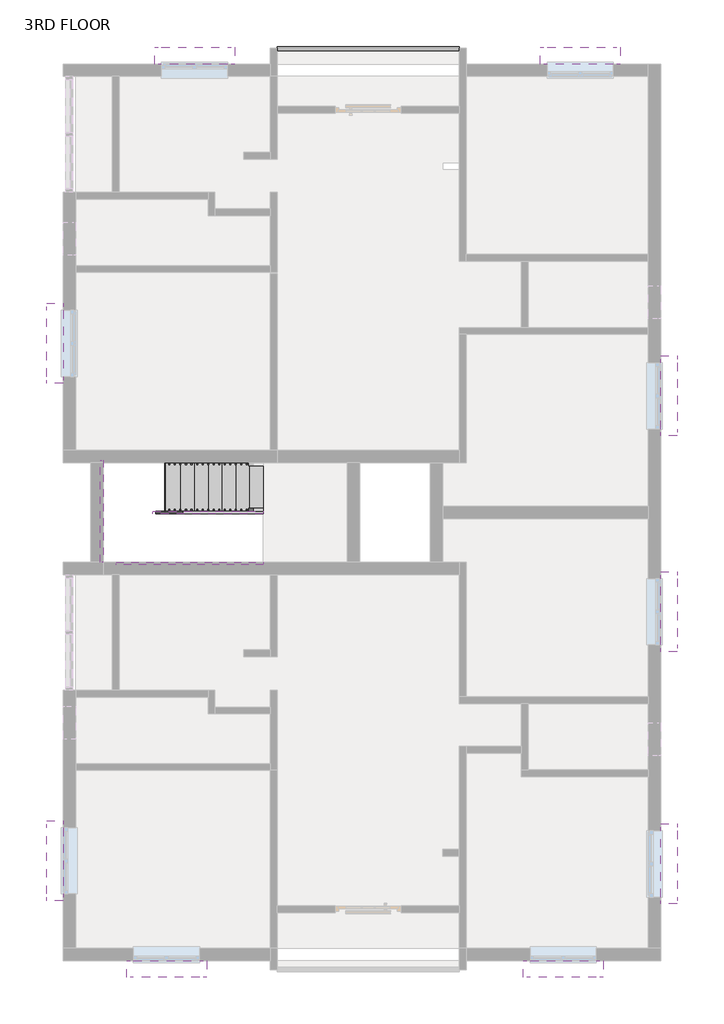
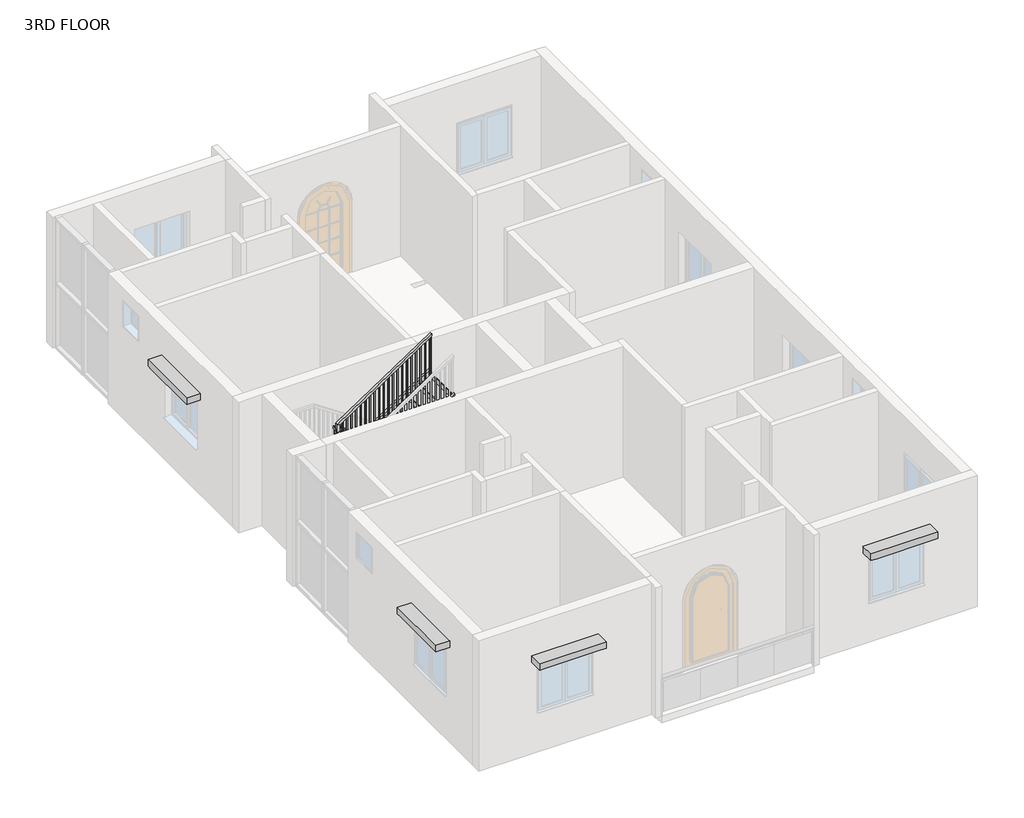
# One storey, part 4 of 4: 9 proxies, 5 members, 2 railings, 1 stair flight.
"""IFC4 building model written with IfcOpenShell, lengths in millimetres."""

from ifc_helpers import new_model, si_unit, point, frame, origin, place, context, project, spatial, polyline, ellipse_curve, trimmed, outline, extrude, faceted_brep, transform, mapped, element, save
from ifc_brep_helpers import plane_surface, extruded_surface, advanced_brep
from components import generic_models_11_generic_models_11_d301a5e8, generic_models_21_generic_models_21_87948dc1, generic_models_1_generic_models_1_fbb7ad13, generic_models_36_generic_models_36_9c63594f, stair_flight_d3eadeea

model = new_model("IFC4")

# Units and contexts
model_context = context("Model", 3, world=origin())
ifc_project = project(units=[si_unit("LENGTHUNIT", "METRE", prefix="MILLI")], contexts=[model_context])

# Site, building, storey
site = spatial("IfcSite", under=ifc_project)
building = spatial("IfcBuilding", under=site)
storey = spatial("IfcBuildingStorey", under=building, Name="3RD FLOOR", Elevation=12192.0)

# Proxies
placement = place(None, origin())
generic_models_11_generic_models_11_shape = generic_models_11_generic_models_11_d301a5e8(model_context)
element("IfcBuildingElementProxy", 1, Name="Generic Models 13 : Generic Models 11", ObjectType="Generic Models 13 : Generic Models 11", at=placement, inside=storey, context=model_context, shape_type="MappedRepresentation", body=[
    mapped(generic_models_11_generic_models_11_shape, transform((0.0, 0.0, -3048.0), x_axis=(1.0, 0.0, 0.0), y_axis=(0.0, 1.0, 0.0), z_axis=(0.0, 0.0, 1.0))),
])
element("IfcBuildingElementProxy", 2, Name="Generic Models 14 : Generic Models 11", ObjectType="Generic Models 14 : Generic Models 11", at=placement, inside=storey, context=model_context, shape_type="MappedRepresentation", body=[
    mapped(generic_models_11_generic_models_11_shape, transform((-7101.0359618, 0.0, -3048.0), x_axis=(1.0, 0.0, 0.0), y_axis=(0.0, 1.0, 0.0), z_axis=(0.0, 0.0, 1.0))),
])
generic_models_21_generic_models_21_shape = generic_models_21_generic_models_21_87948dc1(model_context)
element("IfcBuildingElementProxy", 3, Name="Generic Models 24 : Generic Models 21", ObjectType="Generic Models 24 : Generic Models 21", at=placement, inside=storey, context=model_context, shape_type="MappedRepresentation", body=[
    mapped(generic_models_21_generic_models_21_shape, transform((0.0, 0.0, -3048.0), x_axis=(1.0, 0.0, 0.0), y_axis=(0.0, 1.0, 0.0), z_axis=(0.0, 0.0, 1.0))),
])
element("IfcBuildingElementProxy", 4, Name="Generic Models 25 : Generic Models 21", ObjectType="Generic Models 25 : Generic Models 21", at=placement, inside=storey, context=model_context, shape_type="MappedRepresentation", body=[
    mapped(generic_models_21_generic_models_21_shape, transform((0.0, 4641.85, -3133.6), x_axis=(1.0, 0.0, 0.0), y_axis=(0.0, 1.0, 0.0), z_axis=(0.0, 0.0, 1.0))),
])
element("IfcBuildingElementProxy", 5, Name="Generic Models 26 : Generic Models 21", ObjectType="Generic Models 26 : Generic Models 21", at=placement, inside=storey, context=model_context, shape_type="MappedRepresentation", body=[
    mapped(generic_models_21_generic_models_21_shape, transform((0.0, 8616.95, -3133.6), x_axis=(1.0, 0.0, 0.0), y_axis=(0.0, 1.0, 0.0), z_axis=(0.0, 0.0, 1.0))),
])
generic_models_1_generic_models_1_shape = generic_models_1_generic_models_1_fbb7ad13(model_context)
element("IfcBuildingElementProxy", 6, Name="Generic Models 3 : Generic Models 1", ObjectType="Generic Models 3 : Generic Models 1", at=placement, inside=storey, context=model_context, shape_type="MappedRepresentation", body=[
    mapped(generic_models_1_generic_models_1_shape, transform((0.0, 0.0, -3048.0), x_axis=(1.0, 0.0, 0.0), y_axis=(0.0, 1.0, 0.0), z_axis=(0.0, 0.0, 1.0))),
])
generic_models_36_generic_models_36_shape = generic_models_36_generic_models_36_9c63594f(model_context)
element("IfcBuildingElementProxy", 7, Name="Generic Models 38 : Generic Models 36", ObjectType="Generic Models 38 : Generic Models 36", at=placement, inside=storey, context=model_context, shape_type="MappedRepresentation", body=[
    mapped(generic_models_36_generic_models_36_shape, transform((0.0, 0.0, -3048.0), x_axis=(1.0, 0.0, 0.0), y_axis=(0.0, 1.0, 0.0), z_axis=(0.0, 0.0, 1.0))),
])
element("IfcBuildingElementProxy", 8, Name="Generic Models 39 : Generic Models 36", ObjectType="Generic Models 39 : Generic Models 36", at=placement, inside=storey, context=model_context, shape_type="MappedRepresentation", body=[
    mapped(generic_models_36_generic_models_36_shape, transform((0.0, -9525.0, -3048.0), x_axis=(1.0, 0.0, 0.0), y_axis=(0.0, 1.0, 0.0), z_axis=(0.0, 0.0, 1.0))),
])
element("IfcBuildingElementProxy", 9, Name="Generic Models 4 : Generic Models 1", ObjectType="Generic Models 4 : Generic Models 1", at=placement, inside=storey, context=model_context, shape_type="MappedRepresentation", body=[
    mapped(generic_models_1_generic_models_1_shape, transform((7304.0875, 0.0, -3048.0), x_axis=(1.0, 0.0, 0.0), y_axis=(0.0, 1.0, 0.0), z_axis=(0.0, 0.0, 1.0))),
])

# Members
element("IfcMember", 10, ObjectType="Stringer - 2\" Width", at=placement, inside=storey, context=model_context, shape_type="SweptSolid", body=[
    extrude(outline(polyline([(12192.0, -2748.0012202), (12410.0398409, -2748.0012202), (13730.8398409, -4729.2012202), (13364.5158313, -4729.2012202), (12192.0, -2970.4274732), (12192.0, -2748.0012202)])), frame((0.0, 4990.8309003, 0.0), z_axis=(0.0, 1.0, 0.0), x_axis=(0.0, 0.0, 1.0)), (0.0, 0.0, 1.0), 50.8),
])
element("IfcMember", 11, ObjectType="Stringer - 2\" Width", at=placement, inside=storey, context=model_context, shape_type="SweptSolid", body=[
    extrude(outline(polyline([(13934.0398409, -4780.0012202), (13567.7158313, -4780.0012202), (14922.382498, -2748.0012202), (15288.7065076, -2748.0012202), (13934.0398409, -4780.0012202)])), frame((0.0, 4990.8309003, 0.0), z_axis=(0.0, 1.0, 0.0), x_axis=(0.0, 0.0, 1.0)), (0.0, 0.0, 1.0), 50.8),
])
element("IfcMember", 12, ObjectType="Stringer - 2\" Width", at=placement, inside=storey, context=model_context, shape_type="SweptSolid", body=[
    extrude(outline(polyline([(12192.0, -2748.0012202), (12410.0398409, -2748.0012202), (13792.2, -4821.2414588), (13792.2, -5370.7274732), (12192.0, -2970.4274732), (12192.0, -2748.0012202)])), frame((0.0, 5930.6309003, 0.0), z_axis=(0.0, 1.0, 0.0), x_axis=(0.0, 0.0, 1.0)), (0.0, 0.0, 1.0), 50.8),
])
element("IfcMember", 13, ObjectType="Stringer - 2\" Width", at=placement, inside=storey, context=model_context, shape_type="SweptSolid", body=[
    extrude(outline(polyline([(-5745.2012202, 5981.4309003), (-5694.4012202, 5981.4309003), (-5694.4012202, 4101.8309003), (-5745.2012202, 4101.8309003), (-5745.2012202, 5981.4309003)])), frame((0.0, 0.0, 13487.4), z_axis=(0.0, 0.0, 1.0), x_axis=(1.0, 0.0, 0.0)), (0.0, 0.0, 1.0), 304.8),
])
element("IfcMember", 14, ObjectType="Stringer - 2\" Width", at=placement, inside=storey, context=model_context, shape_type="SweptSolid", body=[
    extrude(outline(polyline([(13487.4, -4900.4749672), (14922.382498, -2748.0012202), (15288.7065076, -2748.0012202), (13487.4, -5449.9609815), (13487.4, -4900.4749672)])), frame((0.0, 4051.0309003, 0.0), z_axis=(0.0, 1.0, 0.0), x_axis=(0.0, 0.0, 1.0)), (0.0, 0.0, 1.0), 50.8),
])

# Railings
element("IfcRailing", 15, ObjectType="Glass Panel - Bottom Fill 2", at=placement, inside=storey, context=model_context, shape_type="SolidModel", body=[
    advanced_brep(
    [(-2494.0012202, 13593.7910566, 13106.4), (-2494.0012202, 13517.5910566, 13106.4), (858.7987798, 13593.7910566, 13106.4), (858.7987798, 13517.5910566, 13106.4)],
    [
        (0, 1, ellipse_curve(frame((-2494.0012202, 13555.6910566, 13106.4), z_axis=(-1.0, 0.0, 0.0), x_axis=(0.0, -1.0, 0.0)), 38.1, 28.575)),
        (1, 0, ellipse_curve(frame((-2494.0012202, 13555.6910566, 13106.4), z_axis=(-1.0, 0.0, 0.0), x_axis=(0.0, -1.0, 0.0)), 38.1, 28.575)),
        (2, 3, ellipse_curve(frame((858.7987798, 13555.6910566, 13106.4), z_axis=(1.0, 0.0, 0.0), x_axis=(0.0, -1.0, 0.0)), 38.1, 28.575)),
        (3, 2, ellipse_curve(frame((858.7987798, 13555.6910566, 13106.4), z_axis=(1.0, 0.0, 0.0), x_axis=(0.0, -1.0, 0.0)), 38.1, 28.575)),
        (0, 2),
        (3, 1),
    ],
    [
        plane_surface(frame((-2494.0012202, 13555.6910566, 13106.4), z_axis=(-1.0, 0.0, 0.0), x_axis=(0.0, 1.0, 0.0))),
        plane_surface(frame((858.7987798, 13555.6910566, 13106.4), z_axis=(1.0, 0.0, 0.0), x_axis=(0.0, 1.0, 0.0))),
        extruded_surface(trimmed(ellipse_curve(frame((858.7987798, 13555.6910566, 13106.4), z_axis=(-1.0, 0.0, 0.0), x_axis=(0.0, -1.0, 0.0)), 38.1, 28.575), [point((858.7987798, 13593.7910566, 13106.4))], [point((858.7987798, 13517.5910566, 13106.4))], True, "CARTESIAN"), (-3352.7999999999997, 0.0, 0.0), 3352.7999999999997),
        extruded_surface(trimmed(ellipse_curve(frame((858.7987798, 13555.6910566, 13106.4), z_axis=(-1.0, 0.0, 0.0), x_axis=(0.0, -1.0, 0.0)), 38.1, 28.575), [point((858.7987798, 13517.5910566, 13106.4))], [point((858.7987798, 13593.7910566, 13106.4))], True, "CARTESIAN"), (-3352.7999999999997, 0.0, 0.0), 3352.7999999999997),
    ],
    [
        (0, [[1, 2]]),
        (1, [[3, 4]]),
        (2, [[-1, 5, -4, 6]]),
        (3, [[-2, -6, -3, -5]]),
    ],
),
    extrude(outline(polyline([(-4.8012202, 13562.2262136), (807.9987798, 13562.2262136), (807.9987798, 13555.8762136), (-4.8012202, 13555.8762136), (-4.8012202, 13562.2262136)])), frame((0.0, 0.0, 12293.6), z_axis=(0.0, 0.0, 1.0), x_axis=(1.0, 0.0, 0.0)), (0.0, 0.0, 1.0), 711.2),
    extrude(outline(polyline([(-817.6012202, 13562.2262136), (-4.8012202, 13562.2262136), (-4.8012202, 13555.8762136), (-817.6012202, 13555.8762136), (-817.6012202, 13562.2262136)])), frame((0.0, 0.0, 12293.6), z_axis=(0.0, 0.0, 1.0), x_axis=(1.0, 0.0, 0.0)), (0.0, 0.0, 1.0), 711.2),
    extrude(outline(polyline([(-1630.4012202, 13562.2262136), (-817.6012202, 13562.2262136), (-817.6012202, 13555.8762136), (-1630.4012202, 13555.8762136), (-1630.4012202, 13562.2262136)])), frame((0.0, 0.0, 12293.6), z_axis=(0.0, 0.0, 1.0), x_axis=(1.0, 0.0, 0.0)), (0.0, 0.0, 1.0), 711.2),
    extrude(outline(polyline([(-2443.2012202, 13562.2262136), (-1630.4012202, 13562.2262136), (-1630.4012202, 13555.8762136), (-2443.2012202, 13555.8762136), (-2443.2012202, 13562.2262136)])), frame((0.0, 0.0, 12293.6), z_axis=(0.0, 0.0, 1.0), x_axis=(1.0, 0.0, 0.0)), (0.0, 0.0, 1.0), 711.2),
    extrude(outline(polyline([(846.0987798, 13546.1660566), (846.0987798, 13565.2160566), (865.1487798, 13565.2160566), (865.1487798, 13546.1660566), (846.0987798, 13546.1660566)])), frame((0.0, 0.0, 12192.0), z_axis=(0.0, 0.0, 1.0), x_axis=(1.0, 0.0, 0.0)), (0.0, 0.0, 1.0), 885.825),
    extrude(outline(polyline([(-2500.3512202, 13546.1660566), (-2500.3512202, 13565.2160566), (-2481.3012202, 13565.2160566), (-2481.3012202, 13546.1660566), (-2500.3512202, 13546.1660566)])), frame((0.0, 0.0, 12192.0), z_axis=(0.0, 0.0, 1.0), x_axis=(1.0, 0.0, 0.0)), (0.0, 0.0, 1.0), 885.825),
])
element("IfcRailing", 16, ObjectType="Handrail - Rectangular", at=placement, inside=storey, context=model_context, shape_type="SolidModel", body=[
    faceted_brep([(-2748.0012202, 5041.6309003, 13275.7333333), (-2748.0012202, 5041.6309003, 13214.6793317), (-2748.0012202, 5092.4309003, 13214.6793317), (-2748.0012202, 5092.4309003, 13275.7333333), (-4703.8012202, 5041.6309003, 14579.6), (-4754.6012202, 5041.6309003, 14552.4126651), (-4754.6012202, 5092.4309003, 14552.4126651), (-4703.8012202, 5092.4309003, 14579.6), (-4703.8012202, 5041.6309003, 14630.4), (-4754.6012202, 5041.6309003, 14579.6), (-4754.6012202, 5092.4309003, 14579.6), (-4703.8012202, 5092.4309003, 14630.4), (-4780.0012202, 5041.6309003, 14630.4), (-4780.0012202, 5041.6309003, 14579.6), (-4830.8012202, 5092.4309003, 14579.6), (-4830.8012202, 5092.4309003, 14630.4), (-4780.0012202, 4990.8309003, 14630.4), (-4830.8012202, 4990.8309003, 14630.4), (-4830.8012202, 4940.0309003, 14579.6), (-4780.0012202, 4940.0309003, 14579.6)], [[[0, 1, 2, 3]], [[1, 0, 4, 5]], [[2, 1, 5, 6]], [[3, 2, 6, 7]], [[0, 3, 7, 4]], [[5, 4, 8, 9]], [[6, 5, 9, 10]], [[7, 6, 10, 11]], [[4, 7, 11, 8]], [[9, 8, 12, 13]], [[10, 9, 13, 14]], [[11, 10, 14, 15]], [[8, 11, 15, 12]], [[16, 17, 18, 19]], [[13, 12, 16, 19]], [[14, 13, 19, 18]], [[15, 14, 18, 17]], [[12, 15, 17, 16]]]),
    faceted_brep([(-4780.0012202, 4990.8309003, 14630.4), (-4780.0012202, 4940.0309003, 14579.6), (-4830.8012202, 4940.0309003, 14579.6), (-4830.8012202, 4990.8309003, 14630.4), (-4780.0012202, 4990.8309003, 14738.6793317), (-4830.8012202, 4990.8309003, 14765.8666667), (-4830.8012202, 4940.0309003, 14765.8666667), (-4780.0012202, 4940.0309003, 14738.6793317)], [[[0, 1, 2, 3]], [[4, 5, 6, 7]], [[1, 0, 4, 7]], [[2, 1, 7, 6]], [[3, 2, 6, 5]], [[0, 3, 5, 4]]]),
    faceted_brep([(-4830.8012202, 4990.8309003, 14765.8666667), (-4780.0012202, 4990.8309003, 14738.6793317), (-4780.0012202, 4940.0309003, 14738.6793317), (-4830.8012202, 4940.0309003, 14765.8666667), (-2748.0012202, 4990.8309003, 16154.4), (-2748.0012202, 4940.0309003, 16154.4), (-2748.0012202, 4940.0309003, 16093.3459984), (-2748.0012202, 4990.8309003, 16093.3459984)], [[[0, 1, 2, 3]], [[4, 5, 6, 7]], [[1, 0, 4, 7]], [[2, 1, 7, 6]], [[3, 2, 6, 5]], [[0, 3, 5, 4]]]),
    extrude(outline(polyline([(16070.0626651, -2782.9262202), (15070.6666667, -2782.9262202), (15070.6666667, -2763.8762202), (16082.7626651, -2763.8762202), (16070.0626651, -2782.9262202)])), frame((0.0, 4955.9059003, 0.0), z_axis=(0.0, 1.0, 0.0), x_axis=(0.0, 0.0, 1.0)), (0.0, 0.0, 1.0), 19.05),
    extrude(outline(polyline([(16002.3293317, -2884.5262202), (15070.6666667, -2884.5262202), (15070.6666667, -2865.4762202), (16015.0293317, -2865.4762202), (16002.3293317, -2884.5262202)])), frame((0.0, 4955.9059003, 0.0), z_axis=(0.0, 1.0, 0.0), x_axis=(0.0, 0.0, 1.0)), (0.0, 0.0, 1.0), 19.05),
    extrude(outline(polyline([(15934.5959984, -2986.1262202), (15070.6666667, -2986.1262202), (15070.6666667, -2967.0762202), (15947.2959984, -2967.0762202), (15934.5959984, -2986.1262202)])), frame((0.0, 4955.9059003, 0.0), z_axis=(0.0, 1.0, 0.0), x_axis=(0.0, 0.0, 1.0)), (0.0, 0.0, 1.0), 19.05),
    extrude(outline(polyline([(15866.8626651, -3087.7262202), (14901.3333333, -3087.7262202), (14901.3333333, -3068.6762202), (15879.5626651, -3068.6762202), (15866.8626651, -3087.7262202)])), frame((0.0, 4955.9059003, 0.0), z_axis=(0.0, 1.0, 0.0), x_axis=(0.0, 0.0, 1.0)), (0.0, 0.0, 1.0), 19.05),
    extrude(outline(polyline([(15799.1293317, -3189.3262202), (14901.3333333, -3189.3262202), (14901.3333333, -3170.2762202), (15811.8293317, -3170.2762202), (15799.1293317, -3189.3262202)])), frame((0.0, 4955.9059003, 0.0), z_axis=(0.0, 1.0, 0.0), x_axis=(0.0, 0.0, 1.0)), (0.0, 0.0, 1.0), 19.05),
    extrude(outline(polyline([(15731.3959984, -3290.9262202), (14732.0, -3290.9262202), (14732.0, -3271.8762202), (15744.0959984, -3271.8762202), (15731.3959984, -3290.9262202)])), frame((0.0, 4955.9059003, 0.0), z_axis=(0.0, 1.0, 0.0), x_axis=(0.0, 0.0, 1.0)), (0.0, 0.0, 1.0), 19.05),
    extrude(outline(polyline([(15663.6626651, -3392.5262202), (14732.0, -3392.5262202), (14732.0, -3373.4762202), (15676.3626651, -3373.4762202), (15663.6626651, -3392.5262202)])), frame((0.0, 4955.9059003, 0.0), z_axis=(0.0, 1.0, 0.0), x_axis=(0.0, 0.0, 1.0)), (0.0, 0.0, 1.0), 19.05),
    extrude(outline(polyline([(15595.9293317, -3494.1262202), (14732.0, -3494.1262202), (14732.0, -3475.0762202), (15608.6293317, -3475.0762202), (15595.9293317, -3494.1262202)])), frame((0.0, 4955.9059003, 0.0), z_axis=(0.0, 1.0, 0.0), x_axis=(0.0, 0.0, 1.0)), (0.0, 0.0, 1.0), 19.05),
    extrude(outline(polyline([(15528.1959984, -3595.7262202), (14562.6666667, -3595.7262202), (14562.6666667, -3576.6762202), (15540.8959984, -3576.6762202), (15528.1959984, -3595.7262202)])), frame((0.0, 4955.9059003, 0.0), z_axis=(0.0, 1.0, 0.0), x_axis=(0.0, 0.0, 1.0)), (0.0, 0.0, 1.0), 19.05),
    extrude(outline(polyline([(15460.4626651, -3697.3262202), (14562.6666667, -3697.3262202), (14562.6666667, -3678.2762202), (15473.1626651, -3678.2762202), (15460.4626651, -3697.3262202)])), frame((0.0, 4955.9059003, 0.0), z_axis=(0.0, 1.0, 0.0), x_axis=(0.0, 0.0, 1.0)), (0.0, 0.0, 1.0), 19.05),
    extrude(outline(polyline([(15392.7293317, -3798.9262202), (14393.3333333, -3798.9262202), (14393.3333333, -3779.8762202), (15405.4293317, -3779.8762202), (15392.7293317, -3798.9262202)])), frame((0.0, 4955.9059003, 0.0), z_axis=(0.0, 1.0, 0.0), x_axis=(0.0, 0.0, 1.0)), (0.0, 0.0, 1.0), 19.05),
    extrude(outline(polyline([(15324.9959984, -3900.5262202), (14393.3333333, -3900.5262202), (14393.3333333, -3881.4762202), (15337.6959984, -3881.4762202), (15324.9959984, -3900.5262202)])), frame((0.0, 4955.9059003, 0.0), z_axis=(0.0, 1.0, 0.0), x_axis=(0.0, 0.0, 1.0)), (0.0, 0.0, 1.0), 19.05),
    extrude(outline(polyline([(15257.2626651, -4002.1262202), (14393.3333333, -4002.1262202), (14393.3333333, -3983.0762202), (15269.9626651, -3983.0762202), (15257.2626651, -4002.1262202)])), frame((0.0, 4955.9059003, 0.0), z_axis=(0.0, 1.0, 0.0), x_axis=(0.0, 0.0, 1.0)), (0.0, 0.0, 1.0), 19.05),
    extrude(outline(polyline([(15189.5293317, -4103.7262202), (14224.0, -4103.7262202), (14224.0, -4084.6762202), (15202.2293317, -4084.6762202), (15189.5293317, -4103.7262202)])), frame((0.0, 4955.9059003, 0.0), z_axis=(0.0, 1.0, 0.0), x_axis=(0.0, 0.0, 1.0)), (0.0, 0.0, 1.0), 19.05),
    extrude(outline(polyline([(15121.7959984, -4205.3262202), (14224.0, -4205.3262202), (14224.0, -4186.2762202), (15134.4959984, -4186.2762202), (15121.7959984, -4205.3262202)])), frame((0.0, 4955.9059003, 0.0), z_axis=(0.0, 1.0, 0.0), x_axis=(0.0, 0.0, 1.0)), (0.0, 0.0, 1.0), 19.05),
    extrude(outline(polyline([(15054.0626651, -4306.9262202), (14054.6666667, -4306.9262202), (14054.6666667, -4287.8762202), (15066.7626651, -4287.8762202), (15054.0626651, -4306.9262202)])), frame((0.0, 4955.9059003, 0.0), z_axis=(0.0, 1.0, 0.0), x_axis=(0.0, 0.0, 1.0)), (0.0, 0.0, 1.0), 19.05),
    extrude(outline(polyline([(14986.3293317, -4408.5262202), (14054.6666667, -4408.5262202), (14054.6666667, -4389.4762202), (14999.0293317, -4389.4762202), (14986.3293317, -4408.5262202)])), frame((0.0, 4955.9059003, 0.0), z_axis=(0.0, 1.0, 0.0), x_axis=(0.0, 0.0, 1.0)), (0.0, 0.0, 1.0), 19.05),
    extrude(outline(polyline([(14918.5959984, -4510.1262202), (14054.6666667, -4510.1262202), (14054.6666667, -4491.0762202), (14931.2959984, -4491.0762202), (14918.5959984, -4510.1262202)])), frame((0.0, 4955.9059003, 0.0), z_axis=(0.0, 1.0, 0.0), x_axis=(0.0, 0.0, 1.0)), (0.0, 0.0, 1.0), 19.05),
    extrude(outline(polyline([(14850.8626651, -4611.7262202), (13885.3333333, -4611.7262202), (13885.3333333, -4592.6762202), (14863.5626651, -4592.6762202), (14850.8626651, -4611.7262202)])), frame((0.0, 4955.9059003, 0.0), z_axis=(0.0, 1.0, 0.0), x_axis=(0.0, 0.0, 1.0)), (0.0, 0.0, 1.0), 19.05),
    extrude(outline(polyline([(14783.1293317, -4713.3262202), (13885.3333333, -4713.3262202), (13885.3333333, -4694.2762202), (14795.8293317, -4694.2762202), (14783.1293317, -4713.3262202)])), frame((0.0, 4955.9059003, 0.0), z_axis=(0.0, 1.0, 0.0), x_axis=(0.0, 0.0, 1.0)), (0.0, 0.0, 1.0), 19.05),
    extrude(outline(polyline([(-4770.4762202, 5057.5059003), (-4789.5262202, 5057.5059003), (-4789.5262202, 5076.5559003), (-4770.4762202, 5076.5559003), (-4770.4762202, 5057.5059003)])), frame((0.0, 0.0, 13716.0), z_axis=(0.0, 0.0, 1.0), x_axis=(1.0, 0.0, 0.0)), (0.0, 0.0, 1.0), 863.6),
    extrude(outline(polyline([(14507.9626651, -4687.9262202), (13546.6666667, -4687.9262202), (13546.6666667, -4668.8762202), (14495.2626651, -4668.8762202), (14507.9626651, -4687.9262202)])), frame((0.0, 5057.5059003, 0.0), z_axis=(0.0, 1.0, 0.0), x_axis=(0.0, 0.0, 1.0)), (0.0, 0.0, 1.0), 19.05),
    extrude(outline(polyline([(14440.2293317, -4586.3262202), (13546.6666667, -4586.3262202), (13546.6666667, -4567.2762202), (14427.5293317, -4567.2762202), (14440.2293317, -4586.3262202)])), frame((0.0, 5057.5059003, 0.0), z_axis=(0.0, 1.0, 0.0), x_axis=(0.0, 0.0, 1.0)), (0.0, 0.0, 1.0), 19.05),
    extrude(outline(polyline([(14372.4959984, -4484.7262202), (13377.3333333, -4484.7262202), (13377.3333333, -4465.6762202), (14359.7959984, -4465.6762202), (14372.4959984, -4484.7262202)])), frame((0.0, 5057.5059003, 0.0), z_axis=(0.0, 1.0, 0.0), x_axis=(0.0, 0.0, 1.0)), (0.0, 0.0, 1.0), 19.05),
    extrude(outline(polyline([(14304.7626651, -4383.1262202), (13377.3333333, -4383.1262202), (13377.3333333, -4364.0762202), (14292.0626651, -4364.0762202), (14304.7626651, -4383.1262202)])), frame((0.0, 5057.5059003, 0.0), z_axis=(0.0, 1.0, 0.0), x_axis=(0.0, 0.0, 1.0)), (0.0, 0.0, 1.0), 19.05),
    extrude(outline(polyline([(14237.0293317, -4281.5262202), (13377.3333333, -4281.5262202), (13377.3333333, -4262.4762202), (14224.3293317, -4262.4762202), (14237.0293317, -4281.5262202)])), frame((0.0, 5057.5059003, 0.0), z_axis=(0.0, 1.0, 0.0), x_axis=(0.0, 0.0, 1.0)), (0.0, 0.0, 1.0), 19.05),
    extrude(outline(polyline([(14169.2959984, -4179.9262202), (13208.0, -4179.9262202), (13208.0, -4160.8762202), (14156.5959984, -4160.8762202), (14169.2959984, -4179.9262202)])), frame((0.0, 5057.5059003, 0.0), z_axis=(0.0, 1.0, 0.0), x_axis=(0.0, 0.0, 1.0)), (0.0, 0.0, 1.0), 19.05),
    extrude(outline(polyline([(14101.5626651, -4078.3262202), (13208.0, -4078.3262202), (13208.0, -4059.2762202), (14088.8626651, -4059.2762202), (14101.5626651, -4078.3262202)])), frame((0.0, 5057.5059003, 0.0), z_axis=(0.0, 1.0, 0.0), x_axis=(0.0, 0.0, 1.0)), (0.0, 0.0, 1.0), 19.05),
    extrude(outline(polyline([(14033.8293317, -3976.7262202), (13038.6666667, -3976.7262202), (13038.6666667, -3957.6762202), (14021.1293317, -3957.6762202), (14033.8293317, -3976.7262202)])), frame((0.0, 5057.5059003, 0.0), z_axis=(0.0, 1.0, 0.0), x_axis=(0.0, 0.0, 1.0)), (0.0, 0.0, 1.0), 19.05),
    extrude(outline(polyline([(13966.0959984, -3875.1262202), (13038.6666667, -3875.1262202), (13038.6666667, -3856.0762202), (13953.3959984, -3856.0762202), (13966.0959984, -3875.1262202)])), frame((0.0, 5057.5059003, 0.0), z_axis=(0.0, 1.0, 0.0), x_axis=(0.0, 0.0, 1.0)), (0.0, 0.0, 1.0), 19.05),
    extrude(outline(polyline([(13898.3626651, -3773.5262202), (13038.6666667, -3773.5262202), (13038.6666667, -3754.4762202), (13885.6626651, -3754.4762202), (13898.3626651, -3773.5262202)])), frame((0.0, 5057.5059003, 0.0), z_axis=(0.0, 1.0, 0.0), x_axis=(0.0, 0.0, 1.0)), (0.0, 0.0, 1.0), 19.05),
    extrude(outline(polyline([(13830.6293317, -3671.9262202), (12869.3333333, -3671.9262202), (12869.3333333, -3652.8762202), (13817.9293317, -3652.8762202), (13830.6293317, -3671.9262202)])), frame((0.0, 5057.5059003, 0.0), z_axis=(0.0, 1.0, 0.0), x_axis=(0.0, 0.0, 1.0)), (0.0, 0.0, 1.0), 19.05),
    extrude(outline(polyline([(13762.8959984, -3570.3262202), (12869.3333333, -3570.3262202), (12869.3333333, -3551.2762202), (13750.1959984, -3551.2762202), (13762.8959984, -3570.3262202)])), frame((0.0, 5057.5059003, 0.0), z_axis=(0.0, 1.0, 0.0), x_axis=(0.0, 0.0, 1.0)), (0.0, 0.0, 1.0), 19.05),
    extrude(outline(polyline([(13695.1626651, -3468.7262202), (12700.0, -3468.7262202), (12700.0, -3449.6762202), (13682.4626651, -3449.6762202), (13695.1626651, -3468.7262202)])), frame((0.0, 5057.5059003, 0.0), z_axis=(0.0, 1.0, 0.0), x_axis=(0.0, 0.0, 1.0)), (0.0, 0.0, 1.0), 19.05),
    extrude(outline(polyline([(13627.4293317, -3367.1262202), (12700.0, -3367.1262202), (12700.0, -3348.0762202), (13614.7293317, -3348.0762202), (13627.4293317, -3367.1262202)])), frame((0.0, 5057.5059003, 0.0), z_axis=(0.0, 1.0, 0.0), x_axis=(0.0, 0.0, 1.0)), (0.0, 0.0, 1.0), 19.05),
    extrude(outline(polyline([(13559.6959984, -3265.5262202), (12700.0, -3265.5262202), (12700.0, -3246.4762202), (13546.9959984, -3246.4762202), (13559.6959984, -3265.5262202)])), frame((0.0, 5057.5059003, 0.0), z_axis=(0.0, 1.0, 0.0), x_axis=(0.0, 0.0, 1.0)), (0.0, 0.0, 1.0), 19.05),
    extrude(outline(polyline([(13491.9626651, -3163.9262202), (12530.6666667, -3163.9262202), (12530.6666667, -3144.8762202), (13479.2626651, -3144.8762202), (13491.9626651, -3163.9262202)])), frame((0.0, 5057.5059003, 0.0), z_axis=(0.0, 1.0, 0.0), x_axis=(0.0, 0.0, 1.0)), (0.0, 0.0, 1.0), 19.05),
    extrude(outline(polyline([(13424.2293317, -3062.3262202), (12530.6666667, -3062.3262202), (12530.6666667, -3043.2762202), (13411.5293317, -3043.2762202), (13424.2293317, -3062.3262202)])), frame((0.0, 5057.5059003, 0.0), z_axis=(0.0, 1.0, 0.0), x_axis=(0.0, 0.0, 1.0)), (0.0, 0.0, 1.0), 19.05),
    extrude(outline(polyline([(13356.4959984, -2960.7262202), (12361.3333333, -2960.7262202), (12361.3333333, -2941.6762202), (13343.7959984, -2941.6762202), (13356.4959984, -2960.7262202)])), frame((0.0, 5057.5059003, 0.0), z_axis=(0.0, 1.0, 0.0), x_axis=(0.0, 0.0, 1.0)), (0.0, 0.0, 1.0), 19.05),
    extrude(outline(polyline([(13288.7626651, -2859.1262202), (12361.3333333, -2859.1262202), (12361.3333333, -2840.0762202), (13276.0626651, -2840.0762202), (13288.7626651, -2859.1262202)])), frame((0.0, 5057.5059003, 0.0), z_axis=(0.0, 1.0, 0.0), x_axis=(0.0, 0.0, 1.0)), (0.0, 0.0, 1.0), 19.05),
    extrude(outline(polyline([(-4795.8762202, 4974.9559003), (-4795.8762202, 4955.9059003), (-4814.9262202, 4955.9059003), (-4814.9262202, 4974.9559003), (-4795.8762202, 4974.9559003)])), frame((0.0, 0.0, 13716.0), z_axis=(0.0, 0.0, 1.0), x_axis=(1.0, 0.0, 0.0)), (0.0, 0.0, 1.0), 863.6),
    extrude(outline(polyline([(-4795.8762202, 5057.5059003), (-4814.9262202, 5057.5059003), (-4814.9262202, 5076.5559003), (-4795.8762202, 5076.5559003), (-4795.8762202, 5057.5059003)])), frame((0.0, 0.0, 13716.0), z_axis=(0.0, 0.0, 1.0), x_axis=(1.0, 0.0, 0.0)), (0.0, 0.0, 1.0), 863.6),
    extrude(outline(polyline([(16080.6459984, -2767.0512202), (15070.6666667, -2767.0512202), (15070.6666667, -2748.0012202), (16093.3459984, -2748.0012202), (16080.6459984, -2767.0512202)])), frame((0.0, 4955.9059003, 0.0), z_axis=(0.0, 1.0, 0.0), x_axis=(0.0, 0.0, 1.0)), (0.0, 0.0, 1.0), 19.05),
    extrude(outline(polyline([(13227.3793317, -2767.0512202), (12361.3333333, -2767.0512202), (12361.3333333, -2748.0012202), (13214.6793317, -2748.0012202), (13227.3793317, -2767.0512202)])), frame((0.0, 5057.5059003, 0.0), z_axis=(0.0, 1.0, 0.0), x_axis=(0.0, 0.0, 1.0)), (0.0, 0.0, 1.0), 19.05),
])

# Stair flight
stair_flight_shape = stair_flight_d3eadeea(model_context)
element("IfcStairFlight", 17, ObjectType="2\" Tread 1\" Nosing 1/4\" Riser", at=placement, inside=storey, context=model_context, shape_type="MappedRepresentation", body=[
    mapped(stair_flight_shape, transform((0.0, 0.0, 0.0), x_axis=(1.0, 0.0, 0.0), y_axis=(0.0, 1.0, 0.0), z_axis=(0.0, 0.0, 1.0))),
])

save(model, "model.ifc")

# Revit data of these elements
# Type "Glass Panel - Bottom Fill 2"
#   Assembly Code = "C2010400"
#   built-in parameter 1008612 = 0.0416667 (stored number, unit not read)
#   built-in parameter 1008611 = 0.0416667 (stored number, unit not read)
#   built-in parameter 1008609 = 0.333333 (stored number, unit not read)
#   built-in parameter 1008604 = 0.166667 (stored number, unit not read)
#   built-in parameter 1008603 = 0.166667 (stored number, unit not read)
#   Railing Height = 3' - 0"
#   built-in parameter 1008630 = 2
#   built-in parameter 1008610 = 2
#   built-in parameter 1008618 = Baluster - Square : 3/4"
# Type "Handrail - Rectangular"
#   Assembly Code = "C2010400"
#   built-in parameter 1008612 = 0.0416667 (stored number, unit not read)
#   built-in parameter 1008611 = 0.0416667 (stored number, unit not read)
#   built-in parameter 1008609 = 0.333333 (stored number, unit not read)
#   built-in parameter 1008604 = 0.166667 (stored number, unit not read)
#   built-in parameter 1008603 = 0.166667 (stored number, unit not read)
#   Railing Height = 3' - 0"
#   built-in parameter 1008630 = 2
#   built-in parameter 1008610 = 2
#   built-in parameter 1008618 = Baluster - Square : 3/4"
# Element 1 (IfcBuildingElementProxy, "Generic Models 13 : Generic Models 11")
#   Phase Created = New Construction
#   Materials on its faces: "white"
# Element 2 (IfcBuildingElementProxy, "Generic Models 14 : Generic Models 11")
#   Phase Created = New Construction
#   Materials on its faces: "white"
# Element 3 (IfcBuildingElementProxy, "Generic Models 24 : Generic Models 21")
#   Phase Created = New Construction
#   Materials on its faces: "white"
# Element 4 (IfcBuildingElementProxy, "Generic Models 25 : Generic Models 21")
#   Phase Created = New Construction
#   Materials on its faces: "white"
# Element 5 (IfcBuildingElementProxy, "Generic Models 26 : Generic Models 21")
#   Phase Created = New Construction
#   Materials on its faces: "white"
# Element 6 (IfcBuildingElementProxy, "Generic Models 3 : Generic Models 1")
#   Phase Created = New Construction
#   Materials on its faces: "white"
# Element 7 (IfcBuildingElementProxy, "Generic Models 38 : Generic Models 36")
#   Phase Created = New Construction
#   Materials on its faces: "white"
# Element 8 (IfcBuildingElementProxy, "Generic Models 39 : Generic Models 36")
#   Phase Created = New Construction
#   Materials on its faces: "white"
# Element 9 (IfcBuildingElementProxy, "Generic Models 4 : Generic Models 1")
#   Phase Created = New Construction
#   Materials on its faces: "white"
# Elements 10, 11, 12, 13, 14 (IfcMember, "Stringer - 2\" Width")
#   Phase Created = New Construction
# Element 15 (IfcRailing, "Glass Panel - Bottom Fill 2")
#   Phase Created = New Construction
#   Materials on its faces: "Glass"
# Element 16 (IfcRailing, "Handrail - Rectangular")
#   Phase Created = New Construction
# Element 17 (IfcStairFlight, "2\" Tread 1\" Nosing 1/4\" Riser")
#   Phase Created = New Construction
# Materials
#   "white": class "Generic", colour RGB 120 120 120, transparency 0, Cost = 0
#   "Glass": class "Glass", colour RGB 0 128 192, transparency 0.75, Description = "Soda Lime Glass", Cost = 0
